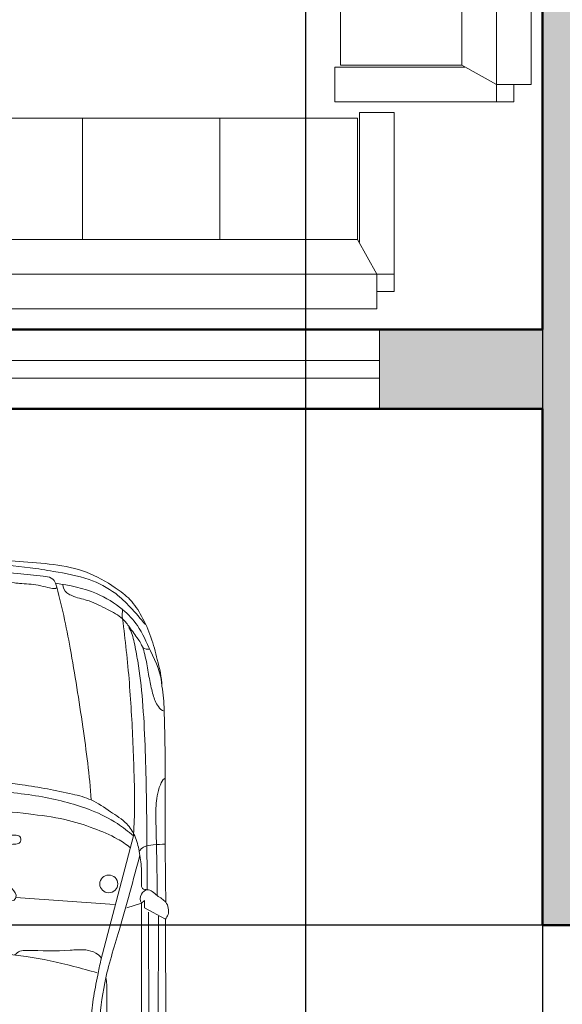
# Model space of a CAD drawing. Units: inches. Extents: x 3398 to 3816, y 15195 to 15771.
# Tile 5 of 10: x 3547 to 3608, y 15306 to 15418. Entities that reach past the tile are written whole.
import ezdxf

# ---------------------------------------------------------------- set-up
doc = ezdxf.new("R2010")
doc.units = ezdxf.units.IN
doc.header["$MEASUREMENT"] = 0
for name, color, linetype, lineweight in [('A-ANNO-DIMS', 2, 'Continuous', 18), ('A-FURN', 8, 'Continuous', 18), ('A-GLAZ', 4, 'Continuous', 18), ('A-WALL', 7, 'Continuous', 50), ('A-WALL-PATT', 252, 'Continuous', 13), ('C-PKNG-VEHI', 8, 'Continuous', 13)]:
    doc.layers.add(name, color=color, linetype=linetype, lineweight=lineweight)
doc.styles.get("Standard").update_dxf_attribs({"font": 'arial.ttf'})
doc.dimstyles.get("Standard").update_dxf_attribs({"dimtxt": 6, "dimasz": 0.18, "dimexe": 0.18, "dimexo": 0.0625, "dimgap": 0.09, "dimtad": 0, "dimtih": 1, "dimtoh": 1, "dimdec": 1, "dimzin": 0, "dimdsep": 46, "dimlunit": 3, "dimtxsty": 'Standard', "dimcen": 0.09, "dimadec": 0, "dimazin": 0, "dimtfac": 1, "dimtdec": 1, "dimtofl": 0, "dimtmove": 0, "dimatfit": 3, "dimfxl": 1, "dimtolj": 1, "dimtzin": 0, "dimarcsym": 0})

# ---------------------------------------------------------------- blocks, each defined once
blk = doc.blocks.new('A$C242571DA')
for p, q in [((1714.3, 1732.5), (3817.1, 1739.9)), ((1659.9, 1632), (1714.3, 1732.5)), ((1699.9, 1699.4), (2984.7, 1695.8)), ((1681.8, 1651.6), (2695.2, 1655.3)), ((1638.3, 1618.5), (1625.1, 1632)), ((1625.1, 1632), (1659.9, 1632)), ((1638.3, 1618.5), (2503.3, 1618.5)), ((1659.9, 1548.1), (1638.3, 1618.5)), ((2503.3, 1618.5), (2861.6, 1607.5)), ((1317.4, 1579.7), (1909.8, 1424.9)), ((3007.2, 1526.5), (2808.1, 1525.2)), ((1644, 1489.1), (1610.4, 1020.2)), ((2311.9, 1454.3), (2500.6, 1456.9)), ((3474.6, 1401.1), (3474.6, 843)), ((4315.2, 1398), (4377.3, 1370.5)), ((1626.1, 1006.5), (1632.8, 719.7)), ((3474.6, 345.6), (3474.6, 903.8)), ((1740.2, 584.9), (1649.3, 586.9)), ((1746.1, 420.6), (1649.3, 420.6)), ((4315.2, 348.7), (4377.3, 376.3)), ((1317.4, 167), (1909.8, 321.9)), ((2311.9, 292.5), (2500.6, 289.8)), ((1659.9, 198.7), (1638.3, 128.2)), ((3007.2, 220.3), (2808.1, 221.6)), ((1638.3, 128.2), (1625.1, 114.7)), ((1625.1, 114.7), (1659.9, 114.7)), ((1638.3, 128.2), (2503.3, 128.2)), ((1659.9, 114.7), (1714.3, 14.2)), ((1681.8, 95.1), (2695.2, 91.4)), ((2503.3, 128.2), (2861.6, 139.2)), ((1699.9, 47.3), (2984.7, 51)), ((1714.3, 14.2), (3817.1, 6.9))]:
    blk.add_line(p, q)
for centre in [(1546.4, 1462.5), (1546.4, 284.2)]:
    blk.add_ellipse(centre, major_axis=(0, 42.9), ratio=0.983266, start_param=4.712389, end_param=10.995574)
for points, knots in [([(1714.3, 1732.5), (1707.7, 1737.6), (1683.3, 1753), (1628.7, 1741.2), (1605.6, 1691.5), (1561.7, 1652.4), (1594.1, 1610.3), (1627.9, 1608.3), (1638.3, 1618.5)], [0, 0, 0, 0, 0.024864, 0.0846267, 0.1362471, 0.1900683, 0.2245199, 0.2681841, 0.2681841, 0.2681841, 0.2681841]), ([(3356.5, 1739.4), (3354.9, 1719.2), (3360.8, 1678.2), (3324, 1631.5), (3255.4, 1544.3), (3187.1, 1476.2), (3125.2, 1432.2)], [0, 0, 0, 0, 0.0597371, 0.1139981, 0.1672498, 0.3938869, 0.3938869, 0.3938869, 0.3938869]), ([(3745.3, 1736.8), (3748.5, 1730.1), (3764.2, 1717.1), (3811.5, 1698.6), (3894.7, 1686.7), (4002.9, 1663.2), (4107.9, 1648.7), (4195.8, 1638.3), (4258.6, 1603.2), (4302.1, 1549.7), (4339.9, 1483.8), (4365.2, 1407.6), (4389.6, 1324.4), (4397.9, 1266.9), (4401.8, 1235.2)], [0, 0, 0, 0, 0.0219205, 0.0572122, 0.1522539, 0.2718866, 0.3894011, 0.4710097, 0.5346344, 0.5986698, 0.6733118, 0.758696, 0.8351341, 0.9293726, 0.9293726, 0.9293726, 0.9293726]), ([(3817.1, 1739.9), (3833.2, 1729.7), (3882.9, 1718.2), (3973.3, 1695.2), (4085.1, 1680.5), (4193.8, 1662.8), (4280.6, 1644.3), (4343.9, 1598.1), (4390, 1540.3), (4427.4, 1448.7), (4457.8, 1336.6), (4475.7, 1233.4), (4478.4, 1175.1), (4479.3, 1161.6)], [0, 0, 0, 0, 0.056668, 0.14946, 0.28161, 0.392935, 0.481686, 0.542967, 0.622845, 0.69797, 0.833643, 0.965665, 1.00577, 1.00577, 1.00577, 1.00577]), ([(0, 873.4), (0, 927.8), (15.6, 1088.6), (25.5, 1309.8), (120.7, 1476.4), (189.2, 1569), (273.5, 1623.1), (369.9, 1666.3), (483, 1694.7), (561.3, 1714.9), (604.6, 1715.7)], [0, 0, 0, 0, 0.16039, 0.479033, 0.632967, 0.722015, 0.817474, 0.927562, 1.03733, 1.167094, 1.167094, 1.167094, 1.167094]), ([(604.6, 1715.7), (545.5, 1714.5), (448.5, 1664.6), (320.8, 1610.6), (225.4, 1521.2), (147.3, 1390.5), (121.7, 1275.2), (113.6, 1208.7)], [0, 0, 0, 0, 0.1772572, 0.3124951, 0.4151678, 0.5597243, 0.7575412, 0.7575412, 0.7575412, 0.7575412]), ([(722.7, 1726.6), (720.8, 1714.9), (694.5, 1689.9), (643, 1671.8), (573.6, 1655.4), (508.5, 1647), (455.2, 1634.7), (428.7, 1627.3), (416.9, 1624.1)], [0, 0, 0, 0, 0.034703, 0.0959761, 0.1659336, 0.2471559, 0.2929944, 0.3295918, 0.3295918, 0.3295918, 0.3295918]), ([(604.6, 1715.7), (642.1, 1723.4), (788.5, 1729.2), (1039.3, 1732.2), (1344.5, 1729.9), (1542, 1733.1), (1633.8, 1733.7)], [0, 0, 0, 0, 0.114897, 0.437061, 0.754269, 1.029686, 1.029686, 1.029686, 1.029686]), ([(1043.6, 1729.2), (1048.6, 1717.9), (1080.9, 1704.2), (1138.6, 1687.6), (1237.7, 1685.6), (1394.7, 1691.3), (1521.7, 1692.4), (1601.5, 1692.7)], [0, 0, 0, 0, 0.0364992, 0.0923739, 0.1867837, 0.3273982, 0.5667068, 0.5667068, 0.5667068, 0.5667068]), ([(1356.8, 1732.2), (1357.1, 1712.8), (1360, 1678.8), (1363.9, 1630.5), (1383.3, 1613.5), (1391, 1607.2)], [0, 0, 0, 0, 1.462159, 2.651105, 3.386321, 3.386321, 3.386321, 3.386321]), ([(2414.7, 1735), (2424.9, 1723.3), (2447.2, 1698.8), (2461.2, 1657.6), (2468.1, 1629), (2468, 1616.1)], [1.808086, 1.808086, 1.808086, 1.808086, 2.918874, 4.131288, 5.10151, 5.10151, 5.10151, 5.10151]), ([(2984.7, 1695.8), (3051, 1695.6), (3172.1, 1691.3), (3367.4, 1677.6), (3575.2, 1664.3), (3788.2, 1643.6), (3968, 1628.1), (4103.8, 1616.8), (4203.6, 1578.1), (4271.8, 1519.5), (4300.6, 1452.1), (4341.7, 1305.3), (4361.8, 1111.2), (4367.5, 936.8), (4367.5, 873.4)], [0, 0, 0, 0, 0.198873, 0.363323, 0.587433, 0.823543, 1.004622, 1.129816, 1.230113, 1.320655, 1.388577, 1.443334, 1.771447, 1.958652, 1.958652, 1.958652, 1.958652]), ([(426.8, 1656.7), (428.5, 1646.6), (426.9, 1625), (399.8, 1616.6), (368.1, 1593.9), (328, 1564.6), (271.6, 1523.9), (237, 1451.9), (196.2, 1376.7), (183.8, 1314.9), (170, 1279.6), (157.2, 1254.2), (133.3, 1244.4), (118.6, 1242.9)], [0, 0, 0, 0, 0.0304541, 0.0502818, 0.0786089, 0.1479133, 0.1986294, 0.2831705, 0.3780326, 0.4523267, 0.4667809, 0.4902599, 0.5347198, 0.5347198, 0.5347198, 0.5347198]), ([(323.7, 1557.5), (344.8, 1571.9), (400.4, 1585.1), (516, 1606.8), (680.3, 1625.8), (885.4, 1635.7), (1116.8, 1642.2), (1346.1, 1644.2), (1504.7, 1644.7), (1574, 1645.7)], [0, 0, 0, 0, 0.076148, 0.165903, 0.355672, 0.569871, 0.782325, 1.050047, 1.257936, 1.257936, 1.257936, 1.257936]), ([(1574, 1645.7), (1572.9, 1638), (1574.1, 1622), (1559.9, 1618.7), (1555.2, 1617.8)], [0, 0, 0, 0, 0.02274132, 0.03717479, 0.03717479, 0.03717479, 0.03717479]), ([(2695.2, 1655.3), (2829.9, 1655.3), (3041.2, 1651.4), (3351.3, 1630.7), (3527.5, 1623.2), (3626.6, 1612)], [0, 0, 0, 0, 0.4042759, 0.6333827, 0.9326252, 0.9326252, 0.9326252, 0.9326252]), ([(310.7, 1637.3), (282.5, 1613.7), (230.1, 1569.9), (148.7, 1486.2), (84.8, 1361.3), (60, 1219), (32.6, 1054.3), (25.1, 944.9), (25.1, 873.4)], [0, 0, 0, 0, 0.1095129, 0.2035347, 0.3452507, 0.5161382, 0.6275464, 0.8383798, 0.8383798, 0.8383798, 0.8383798]), ([(1555.2, 1617.8), (1527.7, 1617.8), (1472.5, 1620.4), (1392.7, 1608.8), (1318.5, 1591), (1249.4, 1545.5), (1201.4, 1466.7), (1142.8, 1385.7), (1104.8, 1240.4), (1076, 1072.3), (1056.4, 932.4), (1056.4, 873.4)], [0, 0, 0, 0, 0.082256, 0.165174, 0.241383, 0.30939, 0.405348, 0.511507, 0.603349, 0.843635, 1.017671, 1.017671, 1.017671, 1.017671]), ([(3535.9, 1563.1), (3520.1, 1550.9), (3484.4, 1526.1), (3408.2, 1510.9), (3323.4, 1473.1), (3207.9, 1445), (3072.6, 1422.2), (2866.9, 1404.6), (2626.4, 1412.9), (2396.7, 1410.8), (2200.9, 1416.9), (2001.3, 1438.2), (1732.1, 1525.9), (1527.9, 1578.9), (1407.5, 1610.7)], [0, 0, 0, 0, 0.05975, 0.126928, 0.230034, 0.336675, 0.482225, 0.641324, 0.954906, 1.203173, 1.330375, 1.542773, 1.802261, 2.175545, 2.175545, 2.175545, 2.175545]), ([(2424, 1618.7), (2441.5, 1589.9), (2464.2, 1518.9), (2495.4, 1450.9), (2501.6, 1411.3)], [0, 0, 0, 0, 0.1000351, 0.2184418, 0.2184418, 0.2184418, 0.2184418]), ([(2507.7, 1618.4), (2521, 1587.7), (2536.6, 1527.1), (2559.6, 1458.5), (2563.3, 1420.6), (2563.8, 1411.4)], [0, 0, 0, 0, 2.528586, 4.711885, 5.408215, 5.408215, 5.408215, 5.408215]), ([(2861.6, 1607.5), (2921.1, 1607.3), (3047.2, 1600.8), (3191.4, 1602), (3356.6, 1584.1), (3498.3, 1570.6), (3623.2, 1549.4), (3664.1, 1533.3)], [0, 0, 0, 0, 0.1783018, 0.3787173, 0.431954, 0.6762374, 0.8077184, 0.8077184, 0.8077184, 0.8077184]), ([(3248.1, 1545.2), (3226.9, 1550.4), (3176.1, 1562.1), (3113.7, 1592.9), (3052.6, 1605.3), (3010.4, 1578.8), (3010.3, 1545.3), (3010.3, 1515.9), (3033.7, 1500.1), (3052.6, 1465.2), (3078.9, 1443.5), (3084, 1424.4)], [0, 0, 0, 0, 0.0655106, 0.1550445, 0.2094604, 0.2438604, 0.287164, 0.3001388, 0.3275984, 0.3616951, 0.4200969, 0.4200969, 0.4200969, 0.4200969]), ([(3626.6, 1612), (3702.5, 1609.1), (3826.2, 1596.8), (3991.4, 1583.2), (4111.7, 1562.4), (4212.2, 1522.7), (4290.4, 1488), (4300.7, 1447.5)], [0, 0, 0, 0, 0.2277977, 0.3719478, 0.4996814, 0.5863441, 0.709615, 0.709615, 0.709615, 0.709615]), ([(1317.4, 1579.7), (1227.8, 1586.1), (1036, 1584.8), (741.2, 1572.5), (486.1, 1553.3), (333.3, 1534.3), (283.3, 1528.5)], [0, 0, 0, 0, 0.269375, 0.574535, 0.885339, 1.036319, 1.036319, 1.036319, 1.036319]), ([(1317.4, 1579.7), (1296.6, 1555.5), (1247.9, 1494.4), (1177.6, 1350.5), (1124.2, 1137.4), (1105.5, 964.9), (1105.5, 873.4)], [0, 0, 0, 0, 0.0947759, 0.2311242, 0.4700259, 0.7400315, 0.7400315, 0.7400315, 0.7400315]), ([(1372.8, 1563.1), (1357.2, 1545), (1321.6, 1490.1), (1277, 1385.7), (1232.8, 1244.2), (1211.1, 1069.4), (1196.8, 942.4), (1196.8, 873.4)], [0, 0, 0, 0, 0.0708922, 0.1925846, 0.3348457, 0.5072814, 0.7109928, 0.7109928, 0.7109928, 0.7109928]), ([(3319, 1587.1), (3303.3, 1568.1), (3256.9, 1516.7), (3206.7, 1467.3), (3171.4, 1439.5)], [0, 0, 0, 0, 1.868162, 5.271297, 5.271297, 5.271297, 5.271297]), ([(2808.1, 1525.2), (2791.9, 1525.1), (2751.9, 1519.7), (2710.6, 1472.6), (2690, 1431.1), (2690.5, 1409.6)], [0, 0, 0, 0, 0.0486628, 0.1144515, 0.1777721, 0.1777721, 0.1777721, 0.1777721]), ([(3275.5, 1532.8), (3287.5, 1528.3), (3299.8, 1504.9), (3308.4, 1482.5), (3311.7, 1472.6)], [0, 0, 0, 0, 0.983949, 1.771691, 1.771691, 1.771691, 1.771691]), ([(3372.2, 1495.3), (3354.4, 1496.8), (3316, 1494.7), (3291.6, 1525.8), (3275.5, 1532.8)], [0, 0, 0, 0, 0.0535488, 0.1060573, 0.1060573, 0.1060573, 0.1060573]), ([(3664.1, 1533.3), (3687, 1526), (3734.8, 1502.3), (3816.7, 1444.8), (3884.1, 1342.9), (3925.1, 1239.9), (3937.3, 1177), (3940.4, 1157.6)], [0, 0, 0, 0, 0.0720749, 0.1581284, 0.2958089, 0.4262456, 0.4842292, 0.4842292, 0.4842292, 0.4842292]), ([(1909.8, 1424.9), (1933.5, 1418.7), (1995.6, 1407.6), (2094.4, 1385.8), (2211.8, 1377.1), (2419, 1366.9), (2704.7, 1366.5), (3032.7, 1354.2), (3316.2, 1371), (3558.7, 1415.9), (3789.1, 1461.7), (4028.9, 1452.9), (4196.2, 1455.2), (4292.7, 1447.9), (4300.7, 1447.5)], [0, 0, 0, 0, 0.073325, 0.188896, 0.303039, 0.425821, 0.811242, 1.159737, 1.41058, 1.660623, 1.899627, 2.11145, 2.377727, 2.401703, 2.401703, 2.401703, 2.401703]), ([(1997.2, 1450.5), (2039.7, 1454.5), (2126.7, 1451.9), (2219.8, 1454.5), (2287.1, 1456.9), (2305.7, 1434.4), (2313.2, 1419.9), (2315.8, 1413.5)], [0, 0, 0, 0, 3.267856, 6.568708, 7.399663, 8.099385, 8.621705, 8.621705, 8.621705, 8.621705]), ([(1898.5, 1426.2), (1889, 1420.6), (1871, 1397.2), (1856.4, 1345.2), (1867.7, 1233.5), (1864.3, 1132.3), (1863, 1038.5), (1876.9, 1022.3), (1884.5, 1015.7)], [0, 0, 0, 0, 0.842998, 2.122875, 3.997599, 9.174838, 10.012722, 10.751336, 10.751336, 10.751336, 10.751336]), ([(113.6, 1208.7), (215.2, 1238.6), (443.2, 1284.9), (788, 1338.7), (1029.5, 1370.7), (1146.4, 1378.6)], [0, 0, 0, 0, 0.317374, 0.69576, 1.04714, 1.04714, 1.04714, 1.04714]), ([(1969.6, 1407.3), (1960.5, 1369.8), (1927, 1259.1), (1890.9, 1078.4), (1874.3, 933), (1874.3, 864.4)], [0, 0, 0, 0, 0.1139079, 0.3411539, 0.543502, 0.543502, 0.543502, 0.543502]), ([(3231.5, 1368.3), (3240.8, 1356.2), (3253.1, 1315.7), (3271.9, 1240.7), (3297.9, 1127.9), (3310.5, 974.6), (3311.2, 858.3), (3311.6, 794.4)], [0, 0, 0, 0, 0.0451009, 0.1211996, 0.2308505, 0.385263, 0.5739042, 0.5739042, 0.5739042, 0.5739042]), ([(3294.8, 1174.5), (3294.8, 1207.4), (3299.6, 1249.5), (3298.3, 1303.9), (3326.3, 1329), (3363.9, 1320.7), (3399.3, 1329.3), (3422.1, 1315.7), (3430.7, 1297.9), (3438.7, 1234.2), (3439.6, 1174.4), (3434.7, 1112.2), (3418.9, 1102), (3395.9, 1098.6), (3362.6, 1100.9), (3331.1, 1096.6), (3298.8, 1107.6), (3297.3, 1140.3), (3294.8, 1160.9), (3294.8, 1174.5)], [0, 0, 0, 0, 0.0969044, 0.1295913, 0.1506192, 0.1985921, 0.2360698, 0.2557908, 0.2719711, 0.2929882, 0.44406, 0.4519132, 0.4720918, 0.4918599, 0.5228758, 0.5707096, 0.5892096, 0.6145759, 0.654681, 0.654681, 0.654681, 0.654681]), ([(4401.8, 1235.2), (4411.9, 1185.3), (4421.6, 1065.8), (4424.1, 946.5), (4424.1, 878)], [0, 0, 0, 0, 0.1502861, 0.3522699, 0.3522699, 0.3522699, 0.3522699]), ([(113.6, 1208.7), (103.3, 1207), (83.6, 1187.6), (76.5, 1122.2), (68.2, 1017.3), (53.4, 925), (53.4, 873.4)], [0, 0, 0, 0, 0.0314754, 0.0702057, 0.1915753, 0.3439346, 0.3439346, 0.3439346, 0.3439346]), ([(135.5, 1213.1), (139.1, 1211.8), (138.4, 1193.3), (132.6, 1168.3), (118.8, 1111.9), (115.6, 1058.9), (109, 974.6), (102.4, 920.1), (102.4, 873.4)], [0, 0, 0, 0, 0.0114788, 0.0403472, 0.0875838, 0.1755608, 0.1991501, 0.3369659, 0.3369659, 0.3369659, 0.3369659]), ([(3940.4, 1157.6), (3949.9, 1111), (3964.3, 1016.4), (3960.5, 921), (3959.8, 873.4)], [0, 0, 0, 0, 0.140379, 0.2808468, 0.2808468, 0.2808468, 0.2808468]), ([(3339.2, 1099), (3339.1, 1094.8), (3336.4, 1010.6), (3333.2, 926.3), (3330, 846.2)], [11.235438, 11.235438, 11.235438, 11.235438, 11.552536, 17.586883, 17.586883, 17.586883, 17.586883]), ([(1311.3, 873.4), (1311.2, 902.4), (1309.2, 950.9), (1315, 1002.2), (1314.2, 1039.4), (1332.1, 1044.9), (1345.7, 1044.2), (1356.8, 1028.5), (1359.2, 970.2), (1361.5, 917.6), (1362.9, 873.4)], [0, 0, 0, 0, 0.0857277, 0.1381048, 0.1641986, 0.1769751, 0.1890325, 0.2028129, 0.2286049, 0.3592554, 0.3592554, 0.3592554, 0.3592554]), ([(1626.1, 1006.5), (1623.5, 1013), (1603.1, 1029.4), (1559.1, 995), (1523, 951.9), (1480.3, 878.3), (1430.5, 774.3), (1385.5, 658.5), (1343.7, 551.3), (1343, 461.7), (1380.3, 386.9), (1428.2, 329.9), (1480.1, 294.6), (1509.8, 257.4), (1524.8, 232.6), (1528, 222.1)], [0, 0, 0, 0, 0.527288, 1.647451, 3.487558, 5.099073, 7.968657, 12.238313, 14.475187, 16.613757, 18.744202, 20.639343, 22.223389, 23.452731, 24.286529, 24.286529, 24.286529, 24.286529]), ([(3231.5, 378.5), (3240.8, 390.5), (3253.1, 431), (3271.9, 506.1), (3297.9, 618.9), (3310.5, 772.1), (3311.2, 888.4), (3311.6, 952.4)], [0, 0, 0, 0, 0.0451009, 0.1211996, 0.2308505, 0.385263, 0.5739042, 0.5739042, 0.5739042, 0.5739042]), ([(3339.2, 647.8), (3339.1, 652), (3336.4, 736.2), (3333.2, 820.5), (3330, 900.6)], [11.235438, 11.235438, 11.235438, 11.235438, 11.552536, 17.586883, 17.586883, 17.586883, 17.586883]), ([(0, 873.4), (0, 819), (15.6, 658.1), (25.5, 437), (120.7, 270.3), (189.2, 177.8), (273.5, 123.7), (369.9, 80.4), (483, 52), (561.3, 31.9), (604.6, 31)], [0, 0, 0, 0, 0.16039, 0.479033, 0.632967, 0.722015, 0.817474, 0.927562, 1.03733, 1.167094, 1.167094, 1.167094, 1.167094]), ([(310.7, 109.5), (282.5, 133.1), (230.1, 176.9), (148.7, 260.5), (84.8, 385.5), (60, 527.8), (32.6, 692.4), (25.1, 801.9), (25.1, 873.4)], [0, 0, 0, 0, 0.1095129, 0.2035347, 0.3452507, 0.5161382, 0.6275464, 0.8383798, 0.8383798, 0.8383798, 0.8383798]), ([(113.6, 538.1), (103.3, 539.8), (83.6, 559.2), (76.5, 624.5), (68.2, 729.4), (53.4, 821.7), (53.4, 873.4)], [0, 0, 0, 0, 0.0314754, 0.0702057, 0.1915753, 0.3439346, 0.3439346, 0.3439346, 0.3439346]), ([(135.5, 533.6), (139.1, 534.9), (138.4, 553.4), (132.6, 578.4), (118.8, 634.9), (115.6, 687.8), (109, 772.2), (102.4, 826.7), (102.4, 873.4)], [0, 0, 0, 0, 0.0114788, 0.0403472, 0.0875838, 0.1755608, 0.1991501, 0.3369659, 0.3369659, 0.3369659, 0.3369659]), ([(1555.2, 129), (1527.7, 129), (1472.5, 126.3), (1392.7, 138), (1318.5, 155.7), (1249.4, 201.3), (1201.4, 280.1), (1142.8, 361.1), (1104.8, 506.4), (1076, 674.5), (1056.4, 814.4), (1056.4, 873.4)], [0, 0, 0, 0, 0.082256, 0.165174, 0.241383, 0.30939, 0.405348, 0.511507, 0.603349, 0.843635, 1.017671, 1.017671, 1.017671, 1.017671]), ([(1317.4, 167), (1296.6, 191.2), (1247.9, 252.4), (1177.6, 396.3), (1124.2, 609.4), (1105.5, 781.8), (1105.5, 873.4)], [0, 0, 0, 0, 0.0947759, 0.2311242, 0.4700259, 0.7400315, 0.7400315, 0.7400315, 0.7400315]), ([(1372.8, 183.6), (1357.2, 201.8), (1321.6, 256.7), (1277, 361), (1232.8, 502.6), (1211.1, 677.3), (1196.8, 804.3), (1196.8, 873.4)], [0, 0, 0, 0, 0.0708922, 0.1925846, 0.3348457, 0.5072814, 0.7109928, 0.7109928, 0.7109928, 0.7109928]), ([(1311.3, 873.4), (1311.2, 844.3), (1309.2, 795.8), (1315, 744.6), (1314.2, 707.4), (1332.1, 701.9), (1345.7, 702.6), (1356.8, 718.2), (1359.2, 776.6), (1361.5, 829.1), (1362.9, 873.4)], [0, 0, 0, 0, 0.0857277, 0.1381048, 0.1641986, 0.1769751, 0.1890325, 0.2028129, 0.2286049, 0.3592554, 0.3592554, 0.3592554, 0.3592554]), ([(1969.6, 339.5), (1960.5, 377), (1926.9, 487.6), (1892.9, 662.7), (1874.3, 801.8), (1874.3, 864.4)], [0, 0, 0, 0, 0.1139079, 0.3411539, 0.5260188, 0.5260188, 0.5260188, 0.5260188]), ([(2984.7, 51), (3051, 51.1), (3172.1, 55.5), (3367.4, 69.2), (3575.2, 82.5), (3788.2, 103.1), (3968, 118.7), (4103.8, 130), (4203.6, 168.6), (4271.8, 227.3), (4300.6, 294.7), (4341.7, 441.5), (4361.8, 635.5), (4367.5, 809.9), (4367.5, 873.4)], [0, 0, 0, 0, 0.198873, 0.363323, 0.587433, 0.823543, 1.004622, 1.129816, 1.230113, 1.320655, 1.388577, 1.443334, 1.771447, 1.958652, 1.958652, 1.958652, 1.958652]), ([(3940.4, 589.1), (3949.9, 635.7), (3964.3, 730.4), (3960.5, 825.8), (3959.8, 873.4)], [0, 0, 0, 0, 0.140379, 0.2808468, 0.2808468, 0.2808468, 0.2808468]), ([(4401.8, 511.5), (4411.9, 561.5), (4421.6, 681), (4424.1, 800.3), (4424.1, 868.8)], [0, 0, 0, 0, 0.1502861, 0.3522699, 0.3522699, 0.3522699, 0.3522699]), ([(1639.2, 326.1), (1635.3, 323.6), (1629, 318.4), (1613.1, 314.9), (1612, 324.2), (1613.2, 330.4), (1619, 337.5), (1629, 345.7), (1637.9, 366.1), (1649, 404.8), (1656.3, 472.9), (1656.2, 543.1), (1644.6, 610.9), (1623, 651.2), (1615, 684.3), (1598.5, 691.2), (1604, 696.6), (1610.3, 699.7), (1618.8, 698.9), (1625.9, 701.3), (1638.1, 698.6), (1633, 713.4), (1632.8, 719.7)], [0, 0, 0, 0, 0.0138597, 0.0278304, 0.0329137, 0.0379971, 0.0465756, 0.0592704, 0.0762214, 0.1105991, 0.1789801, 0.2766959, 0.3173629, 0.3800771, 0.4110544, 0.4160421, 0.4210284, 0.4277212, 0.4387433, 0.4448131, 0.4508005, 0.4694463, 0.4694463, 0.4694463, 0.4694463]), ([(1740.2, 584.9), (1737.8, 571.7), (1749.5, 644.3), (1766.4, 664.5), (1792.2, 700.2), (1821.5, 709.7), (1853.1, 703.9), (1874, 668.4), (1904.5, 622.6), (1915.6, 557.2), (1915.1, 484.2), (1905.7, 417.6), (1884.9, 362.8), (1859.3, 329.1), (1831.3, 318.1), (1810.8, 322.7), (1792.2, 329.3), (1777.9, 350.3), (1753, 385.9), (1737.9, 465.8), (1728.8, 497.3), (1742.4, 597.6), (1740.2, 584.9)], [0, 0, 0, 0, 0.03969, 0.089634, 0.13125, 0.1542862, 0.1797268, 0.2207266, 0.2680991, 0.3447665, 0.4095645, 0.4843001, 0.541515, 0.5817687, 0.6060665, 0.6262474, 0.6436722, 0.6634686, 0.6988791, 0.7758465, 0.8696394, 0.907731, 0.907731, 0.907731, 0.907731]), ([(1863.4, 685.6), (1863.6, 693.5), (1865.3, 711), (1876.9, 724.5), (1884.5, 731)], [9.436432, 9.436432, 9.436432, 9.436432, 10.012722, 10.751336, 10.751336, 10.751336, 10.751336]), ([(1764.9, 587), (1765.6, 590.8), (1766.4, 595.5), (1768.5, 605.7), (1769.7, 611.3), (1773.4, 626.6), (1775.6, 633), (1779.7, 642.1), (1781.6, 644.9), (1785.7, 650.6), (1787.1, 652.5), (1793, 660.3), (1797.4, 666.2), (1804.2, 673.7), (1806.8, 676.1), (1811.1, 679.4), (1812.9, 680.5), (1816.8, 682.1), (1818.8, 682.7), (1824.4, 683.5), (1828.3, 683.2), (1832.5, 682), (1833.6, 681.5), (1836, 680.2), (1837.9, 678.7), (1842.4, 673.7), (1844.9, 670.1), (1850.3, 661.7), (1853.4, 656.6), (1859.3, 647.3), (1862.1, 642.8), (1868.3, 632.6), (1871.4, 626.9), (1876.7, 615.7), (1878.9, 609.8), (1882.8, 597.4), (1884.4, 590.8), (1888.3, 570.5), (1889.7, 556.1), (1891.2, 527.4), (1891.1, 513.1), (1888.9, 470), (1885.1, 441.2), (1874.3, 404), (1870.6, 393.8), (1863.5, 378.7), (1860.6, 373.4), (1854.4, 363.6), (1851.2, 359.2), (1845, 352.6), (1842, 350.2), (1835.8, 346.4), (1832.6, 345.3), (1828.8, 344.6), (1827.9, 344.6), (1824.6, 344.9), (1822.6, 345.2), (1817.8, 346.4), (1814.9, 347.3), (1810.9, 348.7), (1809.4, 349.4), (1808.3, 350.1), (1808.1, 350.2), (1807.3, 351), (1806.7, 351.6), (1804.7, 354), (1803.1, 356.2), (1799.6, 361.3), (1798, 363.7), (1794.9, 368.2), (1793.4, 370.4), (1789.2, 376.9), (1786.7, 381), (1782.4, 389.3), (1780.5, 393.6), (1776.9, 403), (1775.2, 408), (1770.7, 423.5), (1768.3, 434.2), (1764.9, 450.5), (1763.6, 456.4), (1761.4, 466.8), (1760.4, 471.4), (1758.1, 484.4), (1757.3, 492.6), (1757.5, 510.7), (1757.8, 516.5), (1758.6, 528.4), (1759.1, 534.3), (1761.1, 553.9), (1763.1, 570.6), (1764.4, 581.5), (1764.6, 583), (1764.7, 585), (1764.8, 585.5), (1764.8, 586.5), (1764.8, 586.7), (1764.9, 587)], [0.497033, 0.497033, 0.497033, 0.497033, 0.723444, 0.723444, 0.974636, 0.974636, 1.50964, 1.50964, 2.044645, 2.044645, 2.271061, 2.271061, 2.862376, 2.862376, 3.217654, 3.217654, 3.537253, 3.537253, 3.856852, 3.856852, 4.368613, 4.368613, 4.584627, 4.584627, 4.99269, 4.99269, 5.400753, 5.400753, 5.808816, 5.808816, 6.216879, 6.216879, 6.778716, 6.778716, 7.350371, 7.350371, 7.922025, 7.922025, 9.065335, 9.065335, 10.208644, 10.208644, 12.495263, 12.495263, 13.409896, 13.409896, 13.929088, 13.929088, 14.44828, 14.44828, 14.909885, 14.909885, 15.371489, 15.371489, 15.62524, 15.62524, 15.87899, 15.87899, 16.120875, 16.120875, 16.36276, 16.36276, 16.51635, 16.51635, 16.669941, 16.669941, 16.921521, 16.921521, 17.136676, 17.136676, 17.351831, 17.351831, 17.782142, 17.782142, 18.204974, 18.204974, 18.627807, 18.627807, 19.473473, 19.473473, 19.978923, 19.978923, 20.484372, 20.484372, 21.475119, 21.475119, 21.859144, 21.859144, 22.162884, 22.162884, 22.770362, 22.770362, 22.900493, 22.900493, 22.951221, 22.951221, 22.964298, 22.964298, 22.964298, 22.964298]), ([(1863.7, 379.4), (1862.6, 384.2), (1857.6, 413.7), (1866.5, 501.6), (1865.2, 581.4), (1864.1, 639.5)], [1.749253, 1.749253, 1.749253, 1.749253, 2.122875, 3.997599, 8.307432, 8.307432, 8.307432, 8.307432]), ([(3294.8, 572.3), (3294.8, 539.4), (3299.6, 497.2), (3298.3, 442.9), (3326.3, 417.8), (3363.9, 426), (3399.3, 417.5), (3422.1, 431), (3430.7, 448.9), (3438.7, 512.5), (3439.6, 572.4), (3434.7, 634.6), (3418.9, 644.7), (3395.9, 648.2), (3362.6, 645.9), (3331.1, 650.1), (3298.8, 639.2), (3297.3, 606.5), (3294.8, 585.9), (3294.8, 572.3)], [0, 0, 0, 0, 0.0969044, 0.1295913, 0.1506192, 0.1985921, 0.2360698, 0.2557908, 0.2719711, 0.2929882, 0.44406, 0.4519132, 0.4720918, 0.4918599, 0.5228758, 0.5707096, 0.5892096, 0.6145759, 0.654681, 0.654681, 0.654681, 0.654681]), ([(3664.1, 213.5), (3687, 220.8), (3734.8, 244.4), (3816.7, 302), (3884.1, 403.8), (3925.1, 506.9), (3937.3, 569.7), (3940.4, 589.1)], [0, 0, 0, 0, 0.0720749, 0.1581284, 0.2958089, 0.4262456, 0.4842292, 0.4842292, 0.4842292, 0.4842292]), ([(3817.1, 6.9), (3833.2, 17), (3882.9, 28.6), (3973.3, 51.5), (4085.1, 66.3), (4193.8, 84), (4280.6, 102.4), (4343.9, 148.6), (4390, 206.4), (4427.4, 298), (4457.8, 410.1), (4475.7, 513.3), (4478.4, 571.6), (4479.3, 585.2)], [0, 0, 0, 0, 0.056668, 0.14946, 0.28161, 0.392935, 0.481686, 0.542967, 0.622845, 0.69797, 0.833643, 0.965665, 1.00577, 1.00577, 1.00577, 1.00577]), ([(604.6, 31), (545.5, 32.3), (448.5, 82.2), (320.8, 136.1), (225.4, 225.5), (147.3, 356.2), (121.7, 471.5), (113.6, 538.1)], [0, 0, 0, 0, 0.1772572, 0.3124951, 0.4151678, 0.5597243, 0.7575412, 0.7575412, 0.7575412, 0.7575412]), ([(113.6, 538.1), (215.2, 508.2), (443.2, 461.9), (788, 408.1), (1029.5, 376), (1146.4, 368.2)], [0, 0, 0, 0, 0.317374, 0.69576, 1.04714, 1.04714, 1.04714, 1.04714]), ([(426.8, 90), (428.5, 100.2), (426.9, 121.8), (399.8, 130.1), (368.1, 152.8), (328, 182.2), (271.6, 222.8), (237, 294.9), (196.2, 370.1), (183.8, 431.9), (170, 467.2), (157.2, 492.6), (133.3, 502.4), (118.6, 503.9)], [0, 0, 0, 0, 0.0304541, 0.0502818, 0.0786089, 0.1479133, 0.1986294, 0.2831705, 0.3780326, 0.4523267, 0.4667809, 0.4902599, 0.5347198, 0.5347198, 0.5347198, 0.5347198]), ([(3745.3, 10), (3748.5, 16.7), (3764.2, 29.7), (3811.5, 48.1), (3894.7, 60.1), (4002.9, 83.6), (4107.9, 98), (4195.8, 108.4), (4258.6, 143.5), (4302.1, 197), (4339.9, 262.9), (4365.2, 339.2), (4389.6, 422.4), (4397.9, 479.8), (4401.8, 511.5)], [0, 0, 0, 0, 0.0219205, 0.0572122, 0.1522539, 0.2718866, 0.3894011, 0.4710097, 0.5346344, 0.5986698, 0.6733118, 0.758696, 0.8351341, 0.9293726, 0.9293726, 0.9293726, 0.9293726]), ([(1909.8, 321.9), (1933.5, 328.1), (1995.6, 339.2), (2094.4, 361), (2211.8, 369.6), (2419, 379.8), (2704.7, 380.3), (3032.7, 392.6), (3316.2, 375.8), (3558.7, 330.9), (3789.1, 285.1), (4028.9, 293.9), (4196.2, 291.5), (4292.7, 298.8), (4300.7, 299.2)], [0, 0, 0, 0, 0.073325, 0.188896, 0.303039, 0.425821, 0.811242, 1.159737, 1.41058, 1.660623, 1.899627, 2.11145, 2.377727, 2.401703, 2.401703, 2.401703, 2.401703]), ([(3535.9, 183.7), (3520.1, 195.9), (3484.4, 220.6), (3408.2, 235.8), (3323.4, 273.7), (3207.9, 301.8), (3072.6, 324.6), (2866.9, 342.1), (2626.4, 333.8), (2396.7, 335.9), (2200.9, 329.9), (2001.3, 308.6), (1732.1, 220.8), (1527.9, 167.8), (1407.5, 136)], [0, 0, 0, 0, 0.05975, 0.126928, 0.230034, 0.336675, 0.482225, 0.641324, 0.954906, 1.203173, 1.330375, 1.542773, 1.802261, 2.175545, 2.175545, 2.175545, 2.175545]), ([(1898.5, 320.6), (1889, 326.2), (1880.8, 336.8), (1874.8, 348.3), (1874, 349.7)], [0, 0, 0, 0, 0.8429982, 0.9626806, 0.9626806, 0.9626806, 0.9626806]), ([(1997.2, 296.3), (2039.7, 292.2), (2126.7, 294.9), (2219.8, 292.3), (2287.1, 289.9), (2305.7, 312.3), (2313.2, 326.9), (2315.8, 333.2)], [0, 0, 0, 0, 3.267856, 6.568708, 7.399663, 8.099385, 8.621705, 8.621705, 8.621705, 8.621705]), ([(2424, 128), (2441.5, 156.9), (2464.2, 227.8), (2495.4, 295.8), (2501.6, 335.5)], [0, 0, 0, 0, 0.1000351, 0.2184418, 0.2184418, 0.2184418, 0.2184418]), ([(2507.7, 128.3), (2521, 159.1), (2536.6, 219.7), (2559.6, 288.3), (2563.3, 326.1), (2563.8, 335.3)], [0, 0, 0, 0, 2.528586, 4.711885, 5.408215, 5.408215, 5.408215, 5.408215]), ([(2808.1, 221.6), (2791.9, 221.6), (2751.9, 227.1), (2710.6, 274.2), (2690, 315.7), (2690.5, 337.1)], [0, 0, 0, 0, 0.0486628, 0.1144515, 0.1777721, 0.1777721, 0.1777721, 0.1777721]), ([(3248.1, 201.6), (3226.9, 196.3), (3176.1, 184.7), (3113.7, 153.8), (3052.6, 141.4), (3010.4, 168), (3010.3, 201.5), (3010.3, 230.9), (3033.7, 246.6), (3052.6, 281.6), (3078.9, 303.2), (3084, 322.4)], [0, 0, 0, 0, 0.0655106, 0.1550445, 0.2094604, 0.2438604, 0.287164, 0.3001388, 0.3275984, 0.3616951, 0.4200969, 0.4200969, 0.4200969, 0.4200969]), ([(3356.5, 7.4), (3354.9, 27.5), (3360.8, 68.5), (3324, 115.2), (3255.4, 202.5), (3187.1, 270.5), (3125.2, 314.6)], [0, 0, 0, 0, 0.0597371, 0.1139981, 0.1672498, 0.3938869, 0.3938869, 0.3938869, 0.3938869]), ([(3319, 159.7), (3303.3, 178.6), (3256.9, 230), (3206.7, 279.5), (3171.4, 307.2)], [0, 0, 0, 0, 1.868162, 5.271297, 5.271297, 5.271297, 5.271297]), ([(3626.6, 134.7), (3702.5, 137.7), (3826.2, 149.9), (3991.4, 163.5), (4111.7, 184.4), (4212.2, 224.1), (4290.4, 258.8), (4300.7, 299.2)], [0, 0, 0, 0, 0.2277977, 0.3719478, 0.4996814, 0.5863441, 0.709615, 0.709615, 0.709615, 0.709615]), ([(3275.5, 214), (3287.5, 218.5), (3299.8, 241.9), (3308.4, 264.3), (3311.7, 274.2)], [0, 0, 0, 0, 0.983949, 1.771691, 1.771691, 1.771691, 1.771691]), ([(3372.2, 251.5), (3354.4, 249.9), (3316, 252), (3291.6, 220.9), (3275.5, 214)], [0, 0, 0, 0, 0.0535488, 0.1060573, 0.1060573, 0.1060573, 0.1060573]), ([(1317.4, 167), (1227.8, 160.7), (1036, 161.9), (741.2, 174.2), (486.1, 193.4), (333.3, 212.5), (283.3, 218.3)], [0, 0, 0, 0, 0.269375, 0.574535, 0.885339, 1.036319, 1.036319, 1.036319, 1.036319]), ([(323.7, 189.2), (344.8, 174.9), (400.4, 161.7), (516, 139.9), (680.3, 121), (885.4, 111), (1116.8, 104.5), (1346.1, 102.5), (1504.7, 102), (1574, 101.1)], [0, 0, 0, 0, 0.076148, 0.165903, 0.355672, 0.569871, 0.782325, 1.050047, 1.257936, 1.257936, 1.257936, 1.257936]), ([(2861.6, 139.2), (2921.1, 139.4), (3047.2, 146), (3191.4, 144.8), (3356.6, 162.6), (3498.3, 176.1), (3623.2, 197.4), (3664.1, 213.5)], [0, 0, 0, 0, 0.1783018, 0.3787173, 0.431954, 0.6762374, 0.8077184, 0.8077184, 0.8077184, 0.8077184]), ([(722.7, 20.2), (720.8, 31.8), (694.5, 56.8), (643, 75), (573.6, 91.4), (508.5, 99.8), (455.2, 112.1), (428.7, 119.5), (416.9, 122.6)], [0, 0, 0, 0, 0.034703, 0.0959761, 0.1659336, 0.2471559, 0.2929944, 0.3295918, 0.3295918, 0.3295918, 0.3295918]), ([(1356.8, 14.5), (1357.1, 33.9), (1360, 68), (1363.9, 116.3), (1383.3, 133.2), (1391, 139.5)], [0, 0, 0, 0, 1.462159, 2.651105, 3.386321, 3.386321, 3.386321, 3.386321]), ([(1574, 101.1), (1572.9, 108.7), (1574.1, 124.8), (1559.9, 128), (1555.2, 129)], [0, 0, 0, 0, 0.02274132, 0.03717479, 0.03717479, 0.03717479, 0.03717479]), ([(1714.3, 14.2), (1707.7, 9.2), (1683.3, -6.3), (1628.7, 5.5), (1605.6, 55.3), (1561.7, 94.4), (1594.1, 136.5), (1627.9, 138.5), (1638.3, 128.2)], [0, 0, 0, 0, 0.024864, 0.0846267, 0.1362471, 0.1900683, 0.2245199, 0.2681841, 0.2681841, 0.2681841, 0.2681841]), ([(2414.7, 11.8), (2424.9, 23.5), (2447.2, 48), (2461.2, 89.1), (2468.1, 117.8), (2468, 130.7)], [1.808086, 1.808086, 1.808086, 1.808086, 2.918874, 4.131288, 5.10151, 5.10151, 5.10151, 5.10151]), ([(2695.2, 91.4), (2829.9, 91.5), (3041.2, 95.4), (3351.3, 116.1), (3527.5, 123.5), (3626.6, 134.7)], [0, 0, 0, 0, 0.4042759, 0.6333827, 0.9326252, 0.9326252, 0.9326252, 0.9326252]), ([(1043.6, 17.6), (1048.6, 28.9), (1080.9, 42.6), (1138.6, 59.2), (1237.7, 61.2), (1394.7, 55.4), (1521.7, 54.3), (1601.5, 54.1)], [0, 0, 0, 0, 0.0364992, 0.0923739, 0.1867837, 0.3273982, 0.5667068, 0.5667068, 0.5667068, 0.5667068]), ([(604.6, 31), (642.1, 23.4), (788.5, 17.5), (1039.3, 14.6), (1344.5, 16.8), (1542, 13.6), (1633.8, 13.1)], [0, 0, 0, 0, 0.114897, 0.437061, 0.754269, 1.029686, 1.029686, 1.029686, 1.029686])]:
    blk.add_open_spline(points, degree=3, knots=knots)
for points in [[(283.3, 1528.5), (267.8, 1524.6), (251.4, 1527.5), (235.4, 1528.5)], [(3331.9, 1378.1), (3334.2, 1360.4), (3335.9, 1342.5), (3337.3, 1324.5)], [(4479.3, 1161.6), (4491, 1066.2), (4488, 969.5), (4488, 873.4)], [(4479.3, 585.2), (4491, 680.6), (4488, 777.3), (4488, 873.4)], [(3331.9, 368.6), (3334.2, 386.4), (3335.9, 404.3), (3337.3, 422.2)], [(1646.2, 253.1), (1647.8, 277.5), (1640, 301.6), (1639.2, 326.1)], [(283.3, 218.3), (267.8, 222.1), (251.4, 219.2), (235.4, 218.3)]]:
    blk.add_open_spline(points, degree=3)
blk = doc.blocks.new('SOFA-3-SEAT')
for p, q in [((1.96, 55.04), (22.23, 55.04)), ((1.96, 55.04), (1.96, 53.08)), ((3.92, 55.04), (3.92, 1.96)), ((22.23, 51.12), (22.23, 55.04)), ((0, 53.08), (0, 1.96)), ((3.92, 53.08), (0, 53.08)), ((3.92, 53.08), (7.85, 50.88)), ((7.54, 51.12), (22.23, 51.12)), ((21.58, 50.87), (7.85, 50.87)), ((21.58, 35.31), (7.85, 35.31)), ((21.58, 19.74), (7.85, 19.74)), ((7.85, 4.17), (3.92, 1.96)), ((7.29, 3.92), (22.23, 3.92)), ((22.23, 3.92), (22.23, 0)), ((3.92, 1.96), (0, 1.96)), ((1.96, 1.96), (1.96, 0)), ((1.96, 0), (22.23, 0))]:
    blk.add_line(p, q)
blk.add_lwpolyline([(7.85, 50.88), (7.85, 4.17), (21.58, 4.17), (21.58, 50.87)])
blk = doc.blocks.new('WINDOW-SASH-48IN')
for p, q in [((48, 9), (0, 9)), ((48, 5.5), (0, 5.5)), ((0, 3.5), (48, 3.5)), ((0, 0), (48, 0))]:
    blk.add_line(p, q)
blk = doc.blocks.new('*D39')
at = {"layer": 'A-ANNO-DIMS', "color": 0, "lineweight": -2, "transparency": 16777216}
for p, q in [((3465.19, 15373.46), (3465.19, 15203.29)), ((3606.19, 15373.46), (3606.19, 15203.29)), ((3465.37, 15203.47), (3525.58, 15203.47)), ((3606.01, 15203.47), (3545.8, 15203.47))]:
    blk.add_line(p, q, dxfattribs=at)
at = {"layer": 'A-ANNO-DIMS', "color": 0, "transparency": 16777216}
for points in [[(3465.37, 15203.5), (3465.37, 15203.44), (3465.19, 15203.47)], [(3606.01, 15203.5), (3606.01, 15203.44), (3606.19, 15203.47)]]:
    blk.add_solid(points, dxfattribs=at)
at = {"layer": 'Defpoints', "color": 0, "transparency": 16777216}
for p in [(3465.19, 15373.52), (3606.19, 15373.52), (3606.19, 15203.47)]:
    blk.add_point(p, dxfattribs=at)
at = {"layer": 'A-ANNO-DIMS', "color": 0, "transparency": 16777216, "insert": (3535.69, 15203.47), "char_height": 6, "attachment_point": 5}
blk.add_mtext('\\A1;11\'-9"', dxfattribs=at)
blk = doc.blocks.new('*D40')
at = {"layer": 'A-ANNO-DIMS', "color": 0, "lineweight": -2, "transparency": 16777216}
for p, q in [((3465.13, 15373.52), (3415.96, 15373.52)), ((3416.14, 15373.34), (3416.14, 15347.46)), ((3416.14, 15315.2), (3416.14, 15341.08)), ((3606.13, 15315.02), (3415.96, 15315.02))]:
    blk.add_line(p, q, dxfattribs=at)
at = {"layer": 'A-ANNO-DIMS', "color": 0, "transparency": 16777216}
for points in [[(3416.11, 15373.34), (3416.17, 15373.34), (3416.14, 15373.52)], [(3416.11, 15315.2), (3416.17, 15315.2), (3416.14, 15315.02)]]:
    blk.add_solid(points, dxfattribs=at)
at = {"layer": 'Defpoints', "color": 0, "transparency": 16777216}
for p in [(3416.14, 15373.52), (3465.19, 15373.52), (3606.19, 15315.02)]:
    blk.add_point(p, dxfattribs=at)
at = {"layer": 'A-ANNO-DIMS', "color": 0, "transparency": 16777216, "insert": (3416.14, 15344.27), "char_height": 6, "attachment_point": 5}
blk.add_mtext('\\A1;4\'-10 1/2"', dxfattribs=at)
blk = doc.blocks.new('*D42')
at = {"layer": 'A-ANNO-DIMS', "color": 0, "lineweight": -2, "transparency": 16777216}
for p, q in [((3606.19, 15698.39), (3606.19, 15203.29)), ((3610.7, 15698.39), (3610.7, 15203.29)), ((3606.37, 15203.47), (3610.52, 15203.47)), ((3610.7, 15203.47), (3610.88, 15203.47))]:
    blk.add_line(p, q, dxfattribs=at)
at = {"layer": 'A-ANNO-DIMS', "color": 0, "transparency": 16777216}
for points in [[(3606.37, 15203.5), (3606.37, 15203.44), (3606.19, 15203.47)], [(3610.52, 15203.5), (3610.52, 15203.44), (3610.7, 15203.47)]]:
    blk.add_solid(points, dxfattribs=at)
at = {"layer": 'Defpoints', "color": 0, "transparency": 16777216}
for p in [(3606.19, 15698.45), (3610.7, 15698.45), (3610.7, 15203.47)]:
    blk.add_point(p, dxfattribs=at)
at = {"layer": 'A-ANNO-DIMS', "color": 0, "transparency": 16777216, "insert": (3625.93, 15203.47), "char_height": 6, "attachment_point": 5}
blk.add_mtext('\\A1;0\'-4 1/2"', dxfattribs=at)
blk = doc.blocks.new('*D44')
at = {"layer": 'A-ANNO-DIMS', "color": 0, "lineweight": -2, "transparency": 16777216}
for p, q in [((3508.92, 15642.76), (3508.92, 15203.29)), ((3579.37, 15642.76), (3579.37, 15203.29)), ((3509.1, 15203.47), (3526.76, 15203.47)), ((3579.19, 15203.47), (3561.53, 15203.47))]:
    blk.add_line(p, q, dxfattribs=at)
at = {"layer": 'A-ANNO-DIMS', "color": 0, "transparency": 16777216}
for points in [[(3509.1, 15203.5), (3509.1, 15203.44), (3508.92, 15203.47)], [(3579.19, 15203.5), (3579.19, 15203.44), (3579.37, 15203.47)]]:
    blk.add_solid(points, dxfattribs=at)
at = {"layer": 'Defpoints', "color": 0, "transparency": 16777216}
for p in [(3508.92, 15642.82), (3579.37, 15642.82), (3579.37, 15203.47)]:
    blk.add_point(p, dxfattribs=at)
at = {"layer": 'A-ANNO-DIMS', "color": 0, "transparency": 16777216, "insert": (3544.14, 15203.47), "char_height": 6, "attachment_point": 5}
blk.add_mtext('\\A1;5\'-10 1/2"', dxfattribs=at)

msp = doc.modelspace()

# ---------------------------------------------------------------- hatches: boundary and pattern name
at = {"layer": 'A-WALL-PATT'}
h = msp.add_hatch(color=256, dxfattribs=at)
h.dxf.hatch_style = 1
h.paths.add_polyline_path([(3515.96, 15730.52), (3465.19, 15730.52), (3465.19, 15715.52), (3474.19, 15715.52), (3474.19, 15721.52), (3515.96, 15721.52)])
h.paths.add_polyline_path([(3719.81, 15730.52), (3675.76, 15730.52), (3675.76, 15721.52), (3700.69, 15721.52), (3700.69, 15637.52), (3610.69, 15637.52), (3610.69, 15663.97), (3606.19, 15663.97), (3606.19, 15601.52), (3599.08, 15601.52), (3599.08, 15592.52), (3606.19, 15592.52), (3606.19, 15508.52), (3616.69, 15508.52), (3616.69, 15513.02), (3610.69, 15513.02), (3610.69, 15633.02), (3708.19, 15633.02), (3708.19, 15637.52), (3705.19, 15637.52), (3705.19, 15721.52), (3719.81, 15721.52)])
h.paths.add_polyline_path([(3762.19, 15730.52), (3743.77, 15730.52), (3743.77, 15721.52), (3753.19, 15721.52), (3753.19, 15637.52), (3732.19, 15637.52), (3732.19, 15633.02), (3753.19, 15633.02), (3753.19, 15597.39), (3762.19, 15597.39)])
h.paths.add_polyline_path([(3762.19, 15549.39), (3753.19, 15549.39), (3753.19, 15513.02), (3652.69, 15513.02), (3652.69, 15508.52), (3664.69, 15508.52), (3664.69, 15460.52), (3652.69, 15460.52), (3652.69, 15456.02), (3672.19, 15456.02), (3672.19, 15460.52), (3669.19, 15460.52), (3669.19, 15508.52), (3753.19, 15508.52), (3753.19, 15497.51), (3762.19, 15497.51)])
h.paths.add_polyline_path([(3762.19, 15473.48), (3753.19, 15473.48), (3753.19, 15460.52), (3696.19, 15460.52), (3696.19, 15456.02), (3753.19, 15456.02), (3753.19, 15414.25), (3762.19, 15414.25)])
h.paths.add_polyline_path([(3762.19, 15366.28), (3753.19, 15366.28), (3753.19, 15324.02), (3610.69, 15324.02), (3610.69, 15456.02), (3616.69, 15456.02), (3616.69, 15460.52), (3610.69, 15460.52), (3606.19, 15460.52), (3606.19, 15382.52), (3587.73, 15382.52), (3587.73, 15373.52), (3606.19, 15373.52), (3606.19, 15315.02), (3762.19, 15315.02)])
h.paths.add_polyline_path([(3539.73, 15382.52), (3522.19, 15382.52), (3522.19, 15373.52), (3539.73, 15373.52)])
h.paths.add_polyline_path([(3480.19, 15382.52), (3474.19, 15382.52), (3474.19, 15452.47), (3465.19, 15452.47), (3465.19, 15373.52), (3480.19, 15373.52)])
h.paths.add_polyline_path([(3551.04, 15601.52), (3474.19, 15601.52), (3474.19, 15679.52), (3465.19, 15679.52), (3465.19, 15500.47), (3474.19, 15500.47), (3474.19, 15592.52), (3551.04, 15592.52)])

# ---------------------------------------------------------------- linework, layer by layer
at = {"layer": 'A-GLAZ'}
msp.add_line((3587.73, 15382.52), (3587.73, 15373.52), dxfattribs=at)
at = {"layer": 'A-WALL'}
for p, q in [((3606.19, 15460.52), (3606.19, 15382.52)), ((3522.19, 15382.52), (3606.19, 15382.52)), ((3465.19, 15373.52), (3606.19, 15373.52)), ((3606.19, 15373.52), (3606.19, 15315.02)), ((3606.19, 15315.02), (3762.19, 15315.02))]:
    msp.add_line(p, q, dxfattribs=at)

# ---------------------------------------------------------------- block references
at = {"layer": 'A-FURN', "rotation": 180}
msp.add_blockref('SOFA-3-SEAT', (3604.93, 15463.35), dxfattribs=at)
at = {"layer": 'A-FURN', "extrusion": (0, 0, -1), "zscale": -1, "rotation": 90.00000000000078}
msp.add_blockref('SOFA-3-SEAT', (-3534.37, 15384.88), dxfattribs=at)
at = {"layer": 'A-GLAZ', "rotation": 180}
msp.add_blockref('WINDOW-SASH-48IN', (3587.73, 15382.52), dxfattribs=at)
at = {"layer": 'C-PKNG-VEHI', "xscale": 0.023770210920435, "yscale": 0.023770210920435, "zscale": 0.023770210920435, "rotation": 270}
msp.add_blockref('A$C242571DA', (3522.34, 15356.47), dxfattribs=at)

# ---------------------------------------------------------------- dimensions: what is measured, and where the dimension line sits
at = {"layer": 'A-ANNO-DIMS'}
for base, p1, p2, picture, middle in [((3610.7, 15203.47), (3606.19, 15698.45), (3610.7, 15698.45), '*D42', (3625.93, 15203.47)), ((3579.366, 15203.4706), (3508.9188, 15642.8198), (3579.366, 15642.8198), '*D44', (3544.1424, 15203.4706)), ((3606.19, 15203.47), (3465.19, 15373.52), (3606.19, 15373.52), '*D39', (3535.69, 15203.47))]:
    dim = msp.add_linear_dim(base=base, p1=p1, p2=p2, dimstyle='Standard', override={"dimdec": 1, "dimlfac": 1, "dimrnd": 0, "dimzin": 1, "dimdsep": 46, "dimlunit": 4, "dimfrac": 2}, dxfattribs=at)
    dim.commit()
    dim.dimension.update_dxf_attribs({"geometry": picture, "text_midpoint": middle})
dim = msp.add_linear_dim(base=(3416.14, 15373.52), p1=(3606.19, 15315.02), p2=(3465.19, 15373.52), angle=90, dimstyle='Standard', override={"dimdec": 1, "dimlfac": 1, "dimrnd": 0, "dimzin": 1, "dimdsep": 46, "dimlunit": 4, "dimfrac": 2}, dxfattribs=at)
dim.commit()
dim.dimension.update_dxf_attribs({"geometry": '*D40', "text_midpoint": (3416.14, 15344.27)})

doc.saveas('drawing.dxf')
